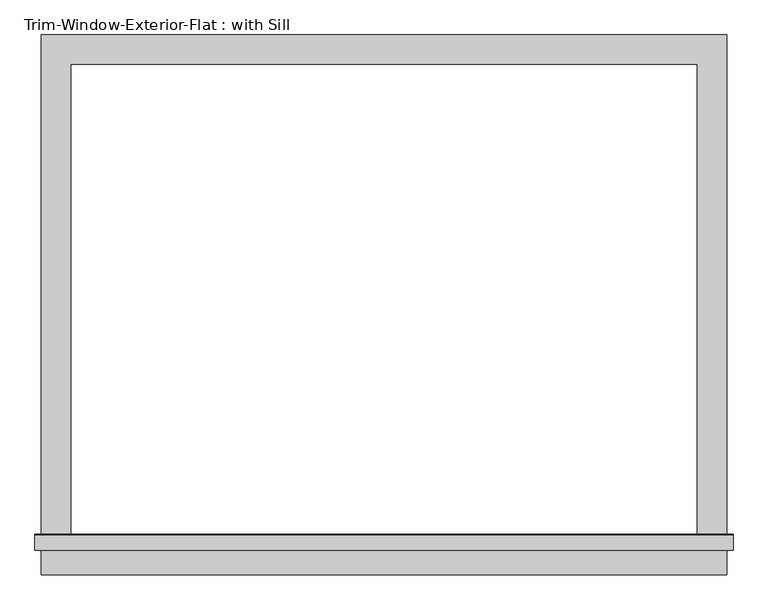
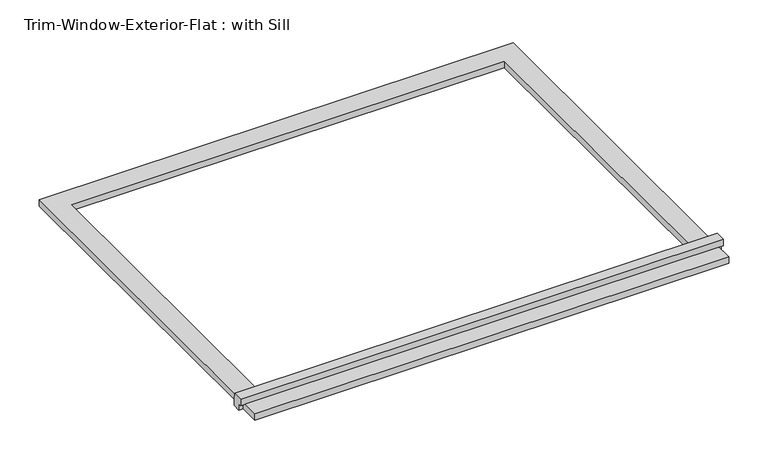
"""IFC4 building model written with IfcOpenShell, lengths in millimetres: proxy geometry, Trim-Window-Exterior-Flat : with Sill."""

from ifc_helpers import new_model, si_unit, frame, origin, origin_with_axes, place, context, project, spatial, polyline, outline, extrude, source, transform, mapped, element, save


def trim_window_exterior_flat_with_sill_c4e67c73(model_context):
    return source(origin(), model_context, "Body", "SweptSolid", [
        extrude(outline(polyline([(666.75, -936.5823709), (666.75, -993.7323709), (-666.75, -993.7323709), (-666.75, -936.5823709), (666.75, -936.5823709)])), origin_with_axes(), (0.0, 0.0, 1.0), 19.05),
        extrude(outline(polyline([(-946.15, 38.1), (-916.8580645, 38.1), (-914.4, 19.05), (-914.4, 0.0), (-936.5823709, 0.0), (-936.5823709, 19.05), (-946.15, 19.05), (-946.15, 38.1)])), frame((-679.45, 0.0, 0.0), z_axis=(1.0, 0.0, 0.0), x_axis=(0.0, 1.0, 0.0)), (0.0, 0.0, 1.0), 1358.9),
        extrude(outline(polyline([(-666.75, 57.15), (666.75, 57.15), (666.75, -914.4), (609.6, -914.4), (609.6, 0.0), (-609.6, 0.0), (-609.6, -914.4), (-666.75, -914.4), (-666.75, 57.15)])), origin_with_axes(), (0.0, 0.0, 1.0), 19.05),
    ])


if __name__ == "__main__":
    model = new_model("IFC4")
    model_context = context("Model", 3, world=origin())
    ifc_project = project(units=[si_unit("LENGTHUNIT", "METRE", prefix="MILLI")], contexts=[model_context])
    site = spatial("IfcSite", under=ifc_project)
    building = spatial("IfcBuilding", under=site)
    placement = place(None, origin())
    trim_window_exterior_flat_with_sill_shape = trim_window_exterior_flat_with_sill_c4e67c73(model_context)
    element("IfcBuildingElementProxy", 1, Name="Trim-Window-Exterior-Flat : with Sill", ObjectType="Trim-Window-Exterior-Flat : with Sill", at=placement, inside=building, context=model_context, shape_type="MappedRepresentation", body=[
        mapped(trim_window_exterior_flat_with_sill_shape, transform((0.0, 0.0, 0.0), x_axis=(1.0, 0.0, 0.0), y_axis=(0.0, 1.0, 0.0), z_axis=(0.0, 0.0, 1.0))),
    ])
    save(model, "model.ifc")

# Revit data of these elements
# Type "Trim-Window-Exterior-Flat : with Sill"
#   Trim Width = 0' - 2 1/4"
#   Trim Thickness_Picture Frame = 0' - 1 1/4"
#   Trim Thickness_with Sill = 0' - 0 3/4"
#   Sill Thickness = 0' - 1 1/4"
#   Opening Width [instance default] = 2' - 0"
#   Opening Height [instance default] = 3' - 0"
#   Default Elevation = 4' - 0"
#   Sill = yes
#   Picture Frame = no
#   Trim Material [instance default] = none
# Element 1 (IfcBuildingElementProxy, "Trim-Window-Exterior-Flat : with Sill")
#   Opening Width = 4' - 0"
#   Trim Material = Clad - White
#   Materials on its faces: "Clad - White"
# Materials
#   "Clad - White": class "Wood", colour RGB 242 242 238, transparency 0, Cost = 0
